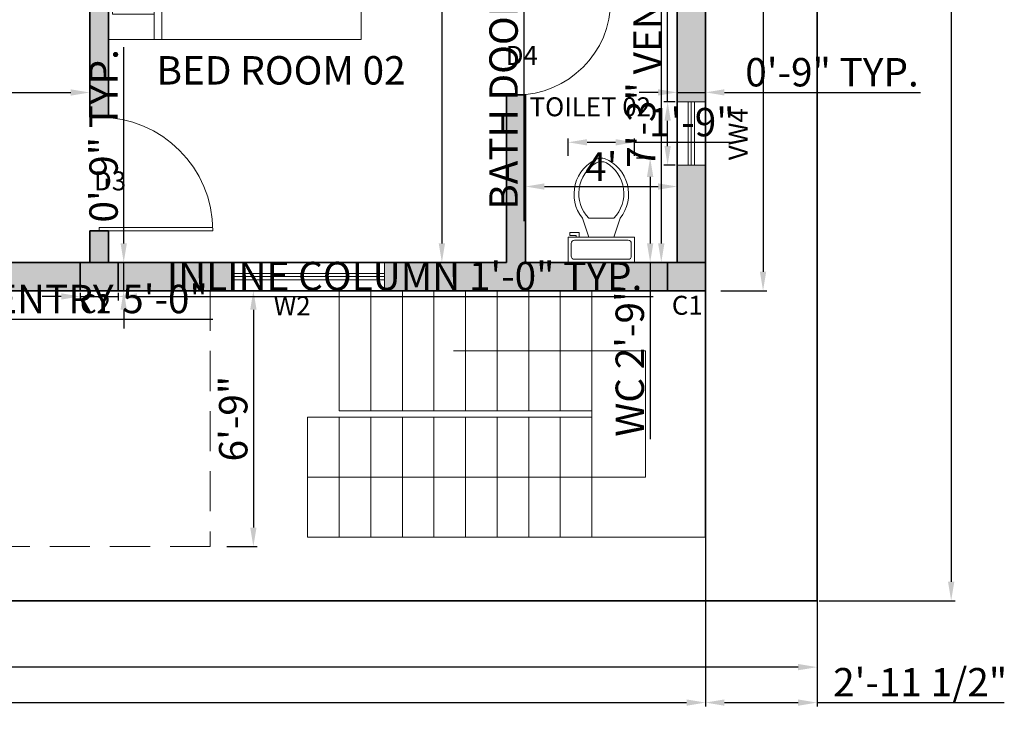
# Model space of a CAD drawing. Units: inches. Extents: x 4312 to 4955, y 6030 to 6717.
# Tile 2 of 5: x 4643 to 4955, y 6030 to 6255. Entities that reach past the tile are written whole.
import ezdxf

# ---------------------------------------------------------------- set-up
doc = ezdxf.new("R2010")
doc.units = ezdxf.units.IN
doc.linetypes.add('DASHED', pattern=[19.05, 12.7, -6.35])
for name, color, linetype, lineweight in [('A-AREA-IDEN', 7, 'Continuous', 20), ('A-FLOR-FIXT', 9, 'Continuous', 18), ('A-FLOR-OVHD', 6, 'DASHED', 13), ('A-WALL', 7, 'Continuous', 35), ('C-PROP', 7, 'Continuous', 35), ('Dimensions', 112, 'Continuous', 13), ('Doors', 10, 'Continuous', 18), ('Furniture', 30, 'Continuous', 18), ('stair case', 130, 'Continuous', 18), ('Text', 30, 'Continuous', 18), ('Windows', 160, 'Continuous', 18)]:
    doc.layers.add(name, color=color, linetype=linetype, lineweight=lineweight)
doc.layers.add('A-WALL-PATT', color=251, linetype='Continuous', lineweight=13, true_color=0x636466)
doc.layers.add('Column', color=52, linetype='Continuous', lineweight=35, true_color=0xc8c92d)
doc.styles.get("Standard").update_dxf_attribs({"font": 'arial.ttf'})
doc.dimstyles.new('ISO-25', dxfattribs={"dimtxt": 9, "dimasz": 6, "dimexe": 1.25, "dimexo": 0.625, "dimtad": 1, "dimdec": 1, "dimlunit": 3, "dimtxsty": 'Standard', "dimcen": 2.5, "dimadec": 0, "dimazin": 0, "dimtfac": 1, "dimtdec": 1, "dimtmove": 0, "dimatfit": 3, "dimfxl": 1, "dimarcsym": 0})

# ---------------------------------------------------------------- blocks, each defined once
blk = doc.blocks.new('D2')
at = {"layer": 'Doors'}
for p, q in [((4718.9, 6093.56), (4754.9, 6093.56)), ((4718.9, 6092.56), (4718.9, 6093.56)), ((4718.9, 6092.56), (4754.9, 6092.56))]:
    blk.add_line(p, q, dxfattribs=at)
blk.add_arc((4718.9, 6092.56), 36, 0, 90, dxfattribs=at)
blk = doc.blocks.new('D3')
at = {"layer": 'Doors'}
for p, q in [((5099.4, 6188.56), (5129.4, 6188.56)), ((5099.4, 6187.72), (5099.4, 6188.56)), ((5099.4, 6187.72), (5129.4, 6187.72))]:
    blk.add_line(p, q, dxfattribs=at)
blk.add_arc((5099.4, 6187.72), 30, 0, 90, dxfattribs=at)
blk = doc.blocks.new('*D17')
at = {"layer": 'Defpoints', "color": 0, "transparency": 16777216}
for p in [(4846.78, 6264.72), (4846.03, 6177.72), (4846.78, 6177.72)]:
    blk.add_point(p, dxfattribs=at)
at = {"layer": 'Dimensions', "color": 0, "lineweight": -2, "transparency": 16777216}
for p, q in [((4846.16, 6264.72), (4844.78, 6264.72)), ((4846.03, 6258.72), (4846.03, 6183.72)), ((4846.16, 6177.72), (4844.78, 6177.72))]:
    blk.add_line(p, q, dxfattribs=at)
at = {"layer": 'Dimensions', "color": 0, "transparency": 16777216}
for points in [[(4845.03, 6258.72), (4847.03, 6258.72), (4846.03, 6264.72)], [(4845.03, 6183.72), (4847.03, 6183.72), (4846.03, 6177.72)]]:
    blk.add_solid(points, dxfattribs=at)
at = {"layer": 'Dimensions', "color": 0, "transparency": 16777216, "insert": (4840.81, 6221.22), "char_height": 9, "attachment_point": 5, "rotation": 90}
blk.add_mtext('7\'-3"', dxfattribs=at)
blk = doc.blocks.new('*D18')
at = {"layer": 'Defpoints', "color": 0, "transparency": 16777216}
for p in [(4803.05, 6207.81), (4851.05, 6207.81), (4851.05, 6201.73)]:
    blk.add_point(p, dxfattribs=at)
at = {"layer": 'Dimensions', "color": 0, "lineweight": -2, "transparency": 16777216}
for p, q in [((4803.05, 6207.19), (4803.05, 6200.48)), ((4851.05, 6207.19), (4851.05, 6200.48)), ((4809.05, 6201.73), (4845.05, 6201.73))]:
    blk.add_line(p, q, dxfattribs=at)
at = {"layer": 'Dimensions', "color": 0, "transparency": 16777216}
for points in [[(4809.05, 6202.73), (4809.05, 6200.73), (4803.05, 6201.73)], [(4845.05, 6202.73), (4845.05, 6200.73), (4851.05, 6201.73)]]:
    blk.add_solid(points, dxfattribs=at)
at = {"layer": 'Dimensions', "color": 0, "transparency": 16777216, "insert": (4827.05, 6206.86), "char_height": 9, "attachment_point": 5}
blk.add_mtext("4'", dxfattribs=at)
blk = doc.blocks.new('*D19')
at = {"layer": 'Defpoints', "color": 0, "transparency": 16777216}
for p in [(4774.62, 6357.72), (4774.62, 6177.72), (4776.57, 6177.72)]:
    blk.add_point(p, dxfattribs=at)
at = {"layer": 'Dimensions', "color": 0, "lineweight": -2, "transparency": 16777216}
for p, q in [((4775.24, 6357.72), (4777.82, 6357.72)), ((4776.57, 6351.72), (4776.57, 6183.72)), ((4775.24, 6177.72), (4777.82, 6177.72))]:
    blk.add_line(p, q, dxfattribs=at)
at = {"layer": 'Dimensions', "color": 0, "transparency": 16777216}
for points in [[(4775.57, 6351.72), (4777.57, 6351.72), (4776.57, 6357.72)], [(4775.57, 6183.72), (4777.57, 6183.72), (4776.57, 6177.72)]]:
    blk.add_solid(points, dxfattribs=at)
at = {"layer": 'Dimensions', "color": 0, "transparency": 16777216, "insert": (4771.35, 6267.72), "char_height": 9, "attachment_point": 5, "rotation": 90}
blk.add_mtext("15'", dxfattribs=at)
blk = doc.blocks.new('*D21')
at = {"layer": 'Defpoints', "color": 0, "transparency": 16777216}
for p in [(4425.05, 6231.5), (4665.05, 6231.5), (4665.05, 6231.5)]:
    blk.add_point(p, dxfattribs=at)
at = {"layer": 'Dimensions', "color": 0, "lineweight": -2, "transparency": 16777216}
for p, q in [((4425.05, 6232.12), (4425.05, 6232.75)), ((4665.05, 6232.12), (4665.05, 6232.75)), ((4431.05, 6231.5), (4659.05, 6231.5))]:
    blk.add_line(p, q, dxfattribs=at)
at = {"layer": 'Dimensions', "color": 0, "transparency": 16777216}
for points in [[(4431.05, 6232.5), (4431.05, 6230.5), (4425.05, 6231.5)], [(4659.05, 6232.5), (4659.05, 6230.5), (4665.05, 6231.5)]]:
    blk.add_solid(points, dxfattribs=at)
at = {"layer": 'Dimensions', "color": 0, "transparency": 16777216, "insert": (4545.05, 6236.72), "char_height": 9, "attachment_point": 5}
blk.add_mtext("20'", dxfattribs=at)
blk = doc.blocks.new('*D25')
at = {"layer": 'Defpoints', "color": 0, "transparency": 16777216}
for p in [(4707.84, 6168.72), (4707.84, 6087.72), (4716.88, 6087.72)]:
    blk.add_point(p, dxfattribs=at)
at = {"layer": 'Dimensions', "color": 0, "lineweight": -2, "transparency": 16777216}
for p, q in [((4708.47, 6168.72), (4718.13, 6168.72)), ((4716.88, 6162.72), (4716.88, 6093.72)), ((4708.47, 6087.72), (4718.13, 6087.72))]:
    blk.add_line(p, q, dxfattribs=at)
at = {"layer": 'Dimensions', "color": 0, "transparency": 16777216}
for points in [[(4715.88, 6162.72), (4717.88, 6162.72), (4716.88, 6168.72)], [(4715.88, 6093.72), (4717.88, 6093.72), (4716.88, 6087.72)]]:
    blk.add_solid(points, dxfattribs=at)
at = {"layer": 'Dimensions', "color": 0, "transparency": 16777216, "insert": (4711.66, 6128.22), "char_height": 9, "attachment_point": 5, "rotation": 90}
blk.add_mtext('6\'-9"', dxfattribs=at)
blk = doc.blocks.new('Toilet - top')
for p, q in [((9.5, -6), (9.5, -2)), ((-10, -8.5), (-8, -8.5)), ((-10, -9.5), (-10, -8.5)), ((-8, -8.5), (-8, -8)), ((-7, -8), (-7, -9.5)), ((-4, -8), (-6, -14)), ((4, -8), (6, -14)), ((-7, -9.5), (-10, -9.5)), ((4, -14), (-4, -14))]:
    blk.add_line(p, q)
blk.add_lwpolyline([(10.5, -8), (10.5, 0), (-10.5, 0), (-10.5, -8)], close=True)
for points in [[(-9.5, -2), (-9.5, -6)], [(8.5, -1), (-8.5, -1)], [(-8.5, -7), (8.5, -7)]]:
    blk.add_lwpolyline(points)
for centre, radius, start, end in [((-8.62, -1.88), 0.884, 81.8699, 188.1301), ((8.62, -1.88), 0.884, 351.8699, 98.1301), ((-8.62, -6.12), 0.884, 171.8699, 278.1301), ((8.62, -6.12), 0.884, 261.8699, 8.1301), ((3.52, -21.58), 12.17, 141.4691, 247.9714), ((4.2, -21.82), 11.33, 136.3677, 238.9468), ((-3.52, -21.58), 12.17, 292.0284, 38.5307), ((-4.2, -21.82), 11.33, 301.053, 43.6321), ((0, -27.88), 4, 245.7318, 294.2682), ((0, -29), 4, 254.8605, 285.1395)]:
    blk.add_arc(centre, radius, start, end)
blk = doc.blocks.new('*D39')
at = {"layer": 'Defpoints', "color": 0, "transparency": 16777216}
for p in [(4857.98, 6552.72), (4864.3, 6168.72), (4878.26, 6168.72)]:
    blk.add_point(p, dxfattribs=at)
at = {"layer": 'Dimensions', "color": 0, "lineweight": -2, "transparency": 16777216}
for p, q in [((4858.6, 6552.72), (4879.51, 6552.72)), ((4878.26, 6546.72), (4878.26, 6174.72)), ((4864.93, 6168.72), (4879.51, 6168.72))]:
    blk.add_line(p, q, dxfattribs=at)
at = {"layer": 'Dimensions', "color": 0, "transparency": 16777216}
for points in [[(4877.26, 6546.72), (4879.26, 6546.72), (4878.26, 6552.72)], [(4877.26, 6174.72), (4879.26, 6174.72), (4878.26, 6168.72)]]:
    blk.add_solid(points, dxfattribs=at)
at = {"layer": 'Dimensions', "color": 0, "transparency": 16777216, "insert": (4873.03, 6360.72), "char_height": 9, "attachment_point": 5, "rotation": 90}
blk.add_mtext("32'", dxfattribs=at)
blk = doc.blocks.new('*D41')
at = {"layer": 'Defpoints', "color": 0, "transparency": 16777216}
for p in [(4895.36, 6639.55), (4895.36, 6070.55), (4937.83, 6070.55)]:
    blk.add_point(p, dxfattribs=at)
at = {"layer": 'Dimensions', "color": 0, "lineweight": -2, "transparency": 16777216}
for p, q in [((4895.99, 6639.55), (4939.08, 6639.55)), ((4937.83, 6633.55), (4937.83, 6076.55)), ((4895.99, 6070.55), (4939.08, 6070.55))]:
    blk.add_line(p, q, dxfattribs=at)
at = {"layer": 'Dimensions', "color": 0, "transparency": 16777216}
for points in [[(4936.83, 6633.55), (4938.83, 6633.55), (4937.83, 6639.55)], [(4936.83, 6076.55), (4938.83, 6076.55), (4937.83, 6070.55)]]:
    blk.add_solid(points, dxfattribs=at)
at = {"layer": 'Dimensions', "color": 0, "transparency": 16777216, "insert": (4931.11, 6355.05), "char_height": 12, "attachment_point": 5, "rotation": 90}
blk.add_mtext('47\'-5"', dxfattribs=at)
blk = doc.blocks.new('*D42')
at = {"layer": 'Defpoints', "color": 0, "transparency": 16777216}
for p in [(4355.36, 6070.55), (4895.36, 6070.55), (4355.36, 6049.53)]:
    blk.add_point(p, dxfattribs=at)
at = {"layer": 'Dimensions', "color": 0, "lineweight": -2, "transparency": 16777216}
for p, q in [((4355.36, 6069.92), (4355.36, 6048.28)), ((4895.36, 6069.92), (4895.36, 6048.28)), ((4889.36, 6049.53), (4361.36, 6049.53))]:
    blk.add_line(p, q, dxfattribs=at)
at = {"layer": 'Dimensions', "color": 0, "transparency": 16777216}
for points in [[(4361.36, 6050.53), (4361.36, 6048.53), (4355.36, 6049.53)], [(4889.36, 6050.53), (4889.36, 6048.53), (4895.36, 6049.53)]]:
    blk.add_solid(points, dxfattribs=at)
at = {"layer": 'Dimensions', "color": 0, "transparency": 16777216, "insert": (4625.36, 6056.26), "char_height": 12, "attachment_point": 5}
blk.add_mtext("45'", dxfattribs=at)
blk = doc.blocks.new('BED-QUEEN-PLAN')
for p, q in [((0, 0), (0, 80.00003)), ((7.99999, 78.80003), (28.79998, 78.80003)), ((7.99999, 65.60003), (7.99999, 78.80003)), ((28.79998, 78.80003), (28.79998, 65.60003)), ((31.19999, 78.80003), (51.99999, 78.80003)), ((31.19999, 65.60003), (31.19999, 78.80003)), ((51.99999, 78.80003), (51.99999, 63.60003)), ((59.99999, 80.00003), (59.99999, 0)), ((0, 65.60003), (44.8, 65.60003)), ((59.99999, 50.40003), (44.8, 65.60003)), ((44.8, 65.60003), (44.8, 50.40003)), ((44.8, 63.20003), (0, 63.20003)), ((51.99999, 63.60003), (46.79936, 63.60003)), ((44.8, 50.40003), (59.99999, 50.40003)), ((59.99999, 0), (0, 0))]:
    blk.add_line(p, q)
blk = doc.blocks.new('VENT-WINDOW-20')
for p, q in [((0, 20), (9, 20)), ((3.5, 20), (3.5, 0)), ((4.5, 20), (4.5, 0)), ((5.5, 20), (5.5, 0)), ((9, 0), (0, 0))]:
    blk.add_line(p, q)
blk = doc.blocks.new('COLUMN-12X9-INLINE')
h = blk.add_hatch(color=256)
h.dxf.hatch_style = 1
h.paths.add_polyline_path([(12, 0), (12, 9), (0, 9), (0, 0)])
for points in [[(0, 0), (0, 9)], [(12, 9), (12, 0)]]:
    blk.add_lwpolyline(points)
blk = doc.blocks.new('*D55')
at = {"layer": 'Defpoints', "color": 0, "transparency": 16777216}
for p in [(4662.02, 6168.72), (4674.02, 6168.72), (4674.02, 6166.92)]:
    blk.add_point(p, dxfattribs=at)
at = {"layer": 'Dimensions', "color": 0, "lineweight": -2, "transparency": 16777216}
for p, q in [((4656.02, 6166.92), (4650.02, 6166.92)), ((4662.02, 6168.1), (4662.02, 6165.67)), ((4662.02, 6166.92), (4674.02, 6166.92)), ((4674.02, 6168.1), (4674.02, 6165.67)), ((4680.02, 6166.92), (4843.47, 6166.92))]:
    blk.add_line(p, q, dxfattribs=at)
at = {"layer": 'Dimensions', "color": 0, "transparency": 16777216}
for points in [[(4656.02, 6167.92), (4656.02, 6165.92), (4662.02, 6166.92)], [(4680.02, 6167.92), (4680.02, 6165.92), (4674.02, 6166.92)]]:
    blk.add_solid(points, dxfattribs=at)
at = {"layer": 'Dimensions', "color": 0, "transparency": 16777216, "insert": (4764.74, 6172.21), "char_height": 9, "attachment_point": 5}
blk.add_mtext('INLINE COLUMN 1\'-0" TYP.', dxfattribs=at)
blk = doc.blocks.new('*D56')
at = {"layer": 'Defpoints', "color": 0, "transparency": 16777216}
for p in [(4674.02, 6177.72), (4675.82, 6177.72), (4674.02, 6168.72)]:
    blk.add_point(p, dxfattribs=at)
at = {"layer": 'Dimensions', "color": 0, "lineweight": -2, "transparency": 16777216}
for p, q in [((4675.82, 6183.72), (4675.82, 6245.83)), ((4674.64, 6177.72), (4677.07, 6177.72)), ((4675.82, 6168.72), (4675.82, 6177.72)), ((4674.64, 6168.72), (4677.07, 6168.72)), ((4675.82, 6162.72), (4675.82, 6156.72))]:
    blk.add_line(p, q, dxfattribs=at)
at = {"layer": 'Dimensions', "color": 0, "transparency": 16777216}
for points in [[(4674.82, 6183.72), (4676.82, 6183.72), (4675.82, 6177.72)], [(4674.82, 6162.72), (4676.82, 6162.72), (4675.82, 6168.72)]]:
    blk.add_solid(points, dxfattribs=at)
at = {"layer": 'Dimensions', "color": 0, "transparency": 16777216, "insert": (4670.6, 6217.78), "char_height": 9, "attachment_point": 5, "rotation": 90}
blk.add_mtext('0\'-9" TYP.', dxfattribs=at)
blk = doc.blocks.new('*D61')
at = {"layer": 'Defpoints', "color": 0, "transparency": 16777216}
for p in [(4807.05, 6360.72), (4802.55, 6330.72), (4807.05, 6330.72)]:
    blk.add_point(p, dxfattribs=at)
at = {"layer": 'Dimensions', "color": 0, "lineweight": -2, "transparency": 16777216}
for p, q in [((4806.42, 6360.72), (4801.3, 6360.72)), ((4802.55, 6354.72), (4802.55, 6336.72)), ((4806.42, 6330.72), (4801.3, 6330.72)), ((4802.55, 6330.72), (4802.55, 6190.78))]:
    blk.add_line(p, q, dxfattribs=at)
at = {"layer": 'Dimensions', "color": 0, "transparency": 16777216}
for points in [[(4801.55, 6354.72), (4803.55, 6354.72), (4802.55, 6360.72)], [(4801.55, 6336.72), (4803.55, 6336.72), (4802.55, 6330.72)]]:
    blk.add_solid(points, dxfattribs=at)
at = {"layer": 'Dimensions', "color": 0, "transparency": 16777216, "insert": (4797.27, 6257.75), "char_height": 9, "attachment_point": 5, "rotation": 90}
blk.add_mtext('BATH DOOR 2\'-6" TYP.', dxfattribs=at)
blk = doc.blocks.new('*D65')
at = {"layer": 'Defpoints', "color": 0, "transparency": 16777216}
for p in [(4848.05, 6228.54), (4851.05, 6228.54), (4851.05, 6208.54)]:
    blk.add_point(p, dxfattribs=at)
at = {"layer": 'Dimensions', "color": 0, "lineweight": -2, "transparency": 16777216}
for p, q in [((4848.05, 6228.54), (4848.05, 6328.15)), ((4850.42, 6228.54), (4846.8, 6228.54)), ((4848.05, 6214.54), (4848.05, 6222.54)), ((4850.42, 6208.54), (4846.8, 6208.54))]:
    blk.add_line(p, q, dxfattribs=at)
at = {"layer": 'Dimensions', "color": 0, "transparency": 16777216}
for points in [[(4847.05, 6222.54), (4849.05, 6222.54), (4848.05, 6228.54)], [(4847.05, 6214.54), (4849.05, 6214.54), (4848.05, 6208.54)]]:
    blk.add_solid(points, dxfattribs=at)
at = {"layer": 'Dimensions', "color": 0, "transparency": 16777216, "insert": (4842.83, 6281.35), "char_height": 9, "attachment_point": 5, "rotation": 90}
blk.add_mtext('VENT 1\'-8" TYP.', dxfattribs=at)
blk = doc.blocks.new('*D66')
at = {"layer": 'Defpoints', "color": 0, "transparency": 16777216}
for p in [(4860.05, 6231.54), (4851.05, 6228.54), (4860.05, 6228.54)]:
    blk.add_point(p, dxfattribs=at)
at = {"layer": 'Dimensions', "color": 0, "lineweight": -2, "transparency": 16777216}
for p, q in [((4851.05, 6229.17), (4851.05, 6232.79)), ((4860.05, 6229.17), (4860.05, 6232.79)), ((4845.05, 6231.54), (4839.05, 6231.54)), ((4851.05, 6231.54), (4860.05, 6231.54)), ((4866.05, 6231.54), (4928.16, 6231.54))]:
    blk.add_line(p, q, dxfattribs=at)
at = {"layer": 'Dimensions', "color": 0, "transparency": 16777216}
for points in [[(4845.05, 6232.54), (4845.05, 6230.54), (4851.05, 6231.54)], [(4866.05, 6232.54), (4866.05, 6230.54), (4860.05, 6231.54)]]:
    blk.add_solid(points, dxfattribs=at)
at = {"layer": 'Dimensions', "color": 0, "transparency": 16777216, "insert": (4900.1, 6236.76), "char_height": 9, "attachment_point": 5}
blk.add_mtext('0\'-9" TYP.', dxfattribs=at)
blk = doc.blocks.new('*D67')
at = {"layer": 'Defpoints', "color": 0, "transparency": 16777216}
for p in [(4567.22, 6168.72), (4627.22, 6168.72), (4627.22, 6159.72)]:
    blk.add_point(p, dxfattribs=at)
at = {"layer": 'Dimensions', "color": 0, "lineweight": -2, "transparency": 16777216}
for p, q in [((4567.22, 6168.1), (4567.22, 6158.47)), ((4627.22, 6168.1), (4627.22, 6158.47)), ((4573.22, 6159.72), (4621.22, 6159.72)), ((4627.22, 6159.72), (4704.03, 6159.72))]:
    blk.add_line(p, q, dxfattribs=at)
at = {"layer": 'Dimensions', "color": 0, "transparency": 16777216}
for points in [[(4573.22, 6160.72), (4573.22, 6158.72), (4567.22, 6159.72)], [(4621.22, 6160.72), (4621.22, 6158.72), (4627.22, 6159.72)]]:
    blk.add_solid(points, dxfattribs=at)
at = {"layer": 'Dimensions', "color": 0, "transparency": 16777216, "insert": (4668.63, 6164.94), "char_height": 9, "attachment_point": 5}
blk.add_mtext('ENTRY 5\'-0"', dxfattribs=at)
blk = doc.blocks.new('*D68')
at = {"layer": 'Defpoints', "color": 0, "transparency": 16777216}
for p in [(4627.22, 6202.22), (4636.22, 6202.22), (4627.22, 6168.72)]:
    blk.add_point(p, dxfattribs=at)
at = {"layer": 'Dimensions', "color": 0, "lineweight": -2, "transparency": 16777216}
for p, q in [((4636.22, 6202.22), (4636.22, 6254.52)), ((4627.85, 6202.22), (4637.47, 6202.22)), ((4636.22, 6174.72), (4636.22, 6196.22)), ((4627.85, 6168.72), (4637.47, 6168.72))]:
    blk.add_line(p, q, dxfattribs=at)
at = {"layer": 'Dimensions', "color": 0, "transparency": 16777216}
for points in [[(4635.22, 6196.22), (4637.22, 6196.22), (4636.22, 6202.22)], [(4635.22, 6174.72), (4637.22, 6174.72), (4636.22, 6168.72)]]:
    blk.add_solid(points, dxfattribs=at)
at = {"layer": 'Dimensions', "color": 0, "transparency": 16777216, "insert": (4630.94, 6231.37), "char_height": 9, "attachment_point": 5, "rotation": 90}
blk.add_mtext('2\'-9 1/2"', dxfattribs=at)
blk = doc.blocks.new('*D85')
at = {"layer": 'Defpoints', "color": 0, "transparency": 16777216}
for p in [(4837.55, 6210.77), (4837.55, 6177.72), (4842.51, 6177.72)]:
    blk.add_point(p, dxfattribs=at)
at = {"layer": 'Dimensions', "color": 0, "lineweight": -2, "transparency": 16777216}
for p, q in [((4838.17, 6210.77), (4843.76, 6210.77)), ((4842.51, 6204.77), (4842.51, 6183.72)), ((4838.17, 6177.72), (4843.76, 6177.72)), ((4842.51, 6177.72), (4842.51, 6121.74))]:
    blk.add_line(p, q, dxfattribs=at)
at = {"layer": 'Dimensions', "color": 0, "transparency": 16777216}
for points in [[(4841.51, 6204.77), (4843.51, 6204.77), (4842.51, 6210.77)], [(4841.51, 6183.72), (4843.51, 6183.72), (4842.51, 6177.72)]]:
    blk.add_solid(points, dxfattribs=at)
at = {"layer": 'Dimensions', "color": 0, "transparency": 16777216, "insert": (4837.23, 6146.73), "char_height": 9, "attachment_point": 5, "rotation": 90}
blk.add_mtext('WC 2\'-9"', dxfattribs=at)
blk = doc.blocks.new('*D86')
at = {"layer": 'Defpoints', "color": 0, "transparency": 16777216}
for p in [(4837.55, 6215.73), (4816.55, 6210.77), (4837.55, 6210.77)]:
    blk.add_point(p, dxfattribs=at)
at = {"layer": 'Dimensions', "color": 0, "lineweight": -2, "transparency": 16777216}
for p, q in [((4816.55, 6211.4), (4816.55, 6216.98)), ((4837.55, 6211.4), (4837.55, 6216.98)), ((4822.55, 6215.73), (4831.55, 6215.73)), ((4837.55, 6215.73), (4867.88, 6215.73))]:
    blk.add_line(p, q, dxfattribs=at)
at = {"layer": 'Dimensions', "color": 0, "transparency": 16777216}
for points in [[(4822.55, 6216.73), (4822.55, 6214.73), (4816.55, 6215.73)], [(4831.55, 6216.73), (4831.55, 6214.73), (4837.55, 6215.73)]]:
    blk.add_solid(points, dxfattribs=at)
at = {"layer": 'Dimensions', "color": 0, "transparency": 16777216, "insert": (4855.71, 6220.95), "char_height": 9, "attachment_point": 5}
blk.add_mtext('1\'-9"', dxfattribs=at)
blk = doc.blocks.new('*D88')
at = {"layer": 'Defpoints', "color": 0, "transparency": 16777216}
for p in [(4895.36, 6639.55), (4860.05, 6552.72), (4895.36, 6038.3)]:
    blk.add_point(p, dxfattribs=at)
at = {"layer": 'Dimensions', "color": 0, "lineweight": -2, "transparency": 16777216}
for p, q in [((4895.36, 6638.92), (4895.36, 6037.05)), ((4860.05, 6552.1), (4860.05, 6037.05)), ((4866.05, 6038.3), (4889.36, 6038.3)), ((4895.36, 6038.3), (4954.65, 6038.3))]:
    blk.add_line(p, q, dxfattribs=at)
at = {"layer": 'Dimensions', "color": 0, "transparency": 16777216}
for points in [[(4866.05, 6039.3), (4866.05, 6037.3), (4860.05, 6038.3)], [(4889.36, 6039.3), (4889.36, 6037.3), (4895.36, 6038.3)]]:
    blk.add_solid(points, dxfattribs=at)
at = {"layer": 'Dimensions', "color": 0, "transparency": 16777216, "insert": (4928.01, 6043.58), "char_height": 9, "attachment_point": 5}
blk.add_mtext('2\'-11 1/2"', dxfattribs=at)
blk = doc.blocks.new('*D89')
at = {"layer": 'Defpoints', "color": 0, "transparency": 16777216}
for p in [(4860.05, 6090.72), (4368.05, 6087.72), (4860.05, 6038.3)]:
    blk.add_point(p, dxfattribs=at)
at = {"layer": 'Dimensions', "color": 0, "lineweight": -2, "transparency": 16777216}
for p, q in [((4860.05, 6090.1), (4860.05, 6037.05)), ((4368.05, 6087.1), (4368.05, 6037.05)), ((4374.05, 6038.3), (4854.05, 6038.3))]:
    blk.add_line(p, q, dxfattribs=at)
at = {"layer": 'Dimensions', "color": 0, "transparency": 16777216}
for points in [[(4374.05, 6039.3), (4374.05, 6037.3), (4368.05, 6038.3)], [(4854.05, 6039.3), (4854.05, 6037.3), (4860.05, 6038.3)]]:
    blk.add_solid(points, dxfattribs=at)
at = {"layer": 'Dimensions', "color": 0, "transparency": 16777216, "insert": (4614.05, 6043.52), "char_height": 9, "attachment_point": 5}
blk.add_mtext('41\'-0"', dxfattribs=at)

msp = doc.modelspace()

# ---------------------------------------------------------------- hatches: boundary and pattern name
at = {"layer": 'A-WALL-PATT'}
h = msp.add_hatch(color=256, dxfattribs=at)
h.dxf.hatch_style = 1
h.paths.add_polyline_path([(4860.05, 6309.06), (4851.05, 6309.06), (4851.05, 6270.72), (4803.05, 6270.72), (4803.05, 6357.72), (4807.05, 6357.72), (4807.05, 6363.72), (4674.05, 6363.72), (4674.05, 6357.72), (4797.05, 6357.72), (4797.05, 6260.72), (4803.05, 6260.72), (4803.05, 6264.72), (4851.05, 6264.72), (4851.05, 6228.54), (4860.05, 6228.54)])
h = msp.add_hatch(color=256, dxfattribs=at)
h.dxf.hatch_style = 1
h.paths.add_polyline_path([(4671.05, 6351.72), (4665.05, 6351.72), (4665.05, 6223.72), (4671.05, 6223.72)])
h = msp.add_hatch(color=256, dxfattribs=at)
h.dxf.hatch_style = 1
h.paths.add_polyline_path([(4848.05, 6177.72), (4803.05, 6177.72), (4803.05, 6230.72), (4797.05, 6230.72), (4797.05, 6177.72), (4758.43, 6177.72), (4758.43, 6168.72), (4848.05, 6168.72)])
h = msp.add_hatch(color=256, dxfattribs=at)
h.dxf.hatch_style = 1
h.paths.add_polyline_path([(4860.05, 6208.54), (4851.05, 6208.54), (4851.05, 6177.72), (4860.05, 6177.72)])
h = msp.add_hatch(color=256, dxfattribs=at)
h.dxf.hatch_style = 1
h.paths.add_polyline_path([(4671.05, 6187.72), (4668.05, 6187.72), (4665.05, 6187.72), (4665.05, 6177.72), (4671.05, 6177.72)])
h = msp.add_hatch(color=256, dxfattribs=at)
h.dxf.hatch_style = 1
h.paths.add_polyline_path([(4662.02, 6177.72), (4627.22, 6177.72), (4627.22, 6168.72), (4662.02, 6168.72)])
h = msp.add_hatch(color=256, dxfattribs=at)
h.dxf.hatch_style = 1
h.paths.add_polyline_path([(4710.44, 6177.72), (4674.02, 6177.72), (4674.02, 6168.72), (4710.44, 6168.72)])
at = {"layer": 'Column'}
h = msp.add_hatch(color=256, dxfattribs=at)
h.dxf.hatch_style = 1
h.paths.add_polyline_path([(4860.05, 6168.72), (4860.05, 6177.72), (4848.05, 6177.72), (4848.05, 6168.72)])

# ---------------------------------------------------------------- linework, layer by layer
at = {"layer": 'A-FLOR-OVHD'}
for p, q in [((4703.23, 6168.72), (4703.23, 6087.72)), ((4703.23, 6087.72), (4368.05, 6087.72))]:
    msp.add_line(p, q, dxfattribs=at)
at = {"layer": 'A-WALL'}
for p, q in [((4860.05, 6552.72), (4860.05, 6090.72)), ((4665.05, 6367.72), (4665.05, 6223.72)), ((4671.05, 6357.72), (4671.05, 6223.72)), ((4851.05, 6264.72), (4851.05, 6177.72)), ((4797.05, 6230.72), (4803.05, 6230.72)), ((4797.05, 6230.72), (4797.05, 6177.72)), ((4803.05, 6230.72), (4803.05, 6177.72)), ((4671.05, 6223.72), (4665.05, 6223.72)), ((4671.05, 6187.72), (4665.05, 6187.72)), ((4665.05, 6187.72), (4665.05, 6177.72)), ((4671.05, 6187.72), (4671.05, 6177.72)), ((4797.05, 6177.72), (4627.22, 6177.72)), ((4797.05, 6177.72), (4671.05, 6177.72)), ((4851.05, 6177.72), (4803.05, 6177.72)), ((4860.05, 6168.72), (4416.05, 6168.72)), ((4860.05, 6168.72), (4627.22, 6168.72))]:
    msp.add_line(p, q, dxfattribs=at)
at = {"layer": 'C-PROP'}
msp.add_lwpolyline([(4895.36, 6639.55), (4895.36, 6070.55), (4355.36, 6070.55), (4379.36, 6639.55)], close=True, dxfattribs=at)
at = {"layer": 'Column'}
msp.add_lwpolyline([(4848.05, 6168.72), (4848.05, 6177.72), (4860.05, 6177.72)], dxfattribs=at)
at = {"layer": 'stair case'}
for p, q in [((4744.05, 6168.72), (4744.05, 6130.72)), ((4754.05, 6168.72), (4754.05, 6130.72)), ((4764.05, 6168.72), (4764.05, 6130.72)), ((4774.05, 6168.72), (4774.05, 6130.72)), ((4784.05, 6168.72), (4784.05, 6130.72)), ((4794.05, 6168.72), (4794.05, 6130.72)), ((4804.05, 6168.72), (4804.05, 6130.72)), ((4814.05, 6168.72), (4814.05, 6130.72)), ((4824.05, 6168.72), (4824.05, 6090.72)), ((4841.01, 6149.72), (4780.25, 6149.72)), ((4841.01, 6149.72), (4841.01, 6109.72)), ((4824.05, 6130.72), (4744.05, 6130.72)), ((4734.05, 6128.72), (4734.05, 6090.72)), ((4824.05, 6128.72), (4734.05, 6128.72)), ((4744.05, 6128.72), (4744.05, 6090.72)), ((4754.05, 6128.72), (4754.05, 6090.72)), ((4764.05, 6128.72), (4764.05, 6090.72)), ((4774.05, 6128.72), (4774.05, 6090.72)), ((4784.05, 6128.72), (4784.05, 6090.72)), ((4794.05, 6128.72), (4794.05, 6090.72)), ((4804.05, 6128.72), (4804.05, 6090.72)), ((4814.05, 6128.72), (4814.05, 6090.72)), ((4734.05, 6109.72), (4841.01, 6109.72)), ((4734.05, 6090.72), (4860.05, 6090.72))]:
    msp.add_line(p, q, dxfattribs=at)
at = {"layer": 'Windows'}
for p, q in [((4710.44, 6168.72), (4710.44, 6177.72)), ((4758.43, 6177.72), (4758.43, 6168.72)), ((4710.43, 6174.22), (4758.43, 6174.22)), ((4710.43, 6173.22), (4758.43, 6173.22)), ((4710.43, 6172.22), (4758.43, 6172.22))]:
    msp.add_line(p, q, dxfattribs=at)

# ---------------------------------------------------------------- block references
at = {"layer": 'A-FLOR-FIXT', "xscale": -1, "rotation": 180}
msp.add_blockref('Toilet - top', (4827.05, 6177.72), dxfattribs=at)
at = {"layer": 'Column'}
msp.add_blockref('COLUMN-12X9-INLINE', (4662.02, 6168.72), dxfattribs=at)
at = {"layer": 'Doors', "xscale": -1, "rotation": 180}
msp.add_blockref('D3', (-299.35, 12448.45), dxfattribs=at)
at = {"layer": 'Doors'}
msp.add_blockref('D2', (-50.85, 95.16), dxfattribs=at)
at = {"layer": 'Furniture', "rotation": 90.00000000000134}
msp.add_blockref('BED-QUEEN-PLAN', (4751.05, 6248.3), dxfattribs=at)
at = {"layer": 'Windows'}
msp.add_blockref('VENT-WINDOW-20', (4851.05, 6208.54), dxfattribs=at)

# ---------------------------------------------------------------- texts
at = {"layer": 'A-AREA-IDEN', "attachment_point": 1, "rotation": 0.0025}
for s, width, insert, char_height in [('BED ROOM 02', 89.0701, (4686.22, 6243.02), 9), ('TOILET 02', 65.4832, (4804.33, 6229.98), 6)]:
    msp.add_mtext_dynamic_manual_height_columns(s, width=width, gutter_width=12.5, heights=[0], dxfattribs=dict(at, insert=insert, char_height=char_height))
at = {"layer": 'Text', "char_height": 6, "attachment_point": 1}
for s, insert in [('D4', (4796.78, 6246.25)), ('D3', (4666.42, 6206.5)), ('C2', (4662.01, 6167.61)), ('W2', (4723.29, 6166.97)), ('C1', (4849.38, 6167.12))]:
    msp.add_mtext_dynamic_manual_height_columns(s, width=4.4911, gutter_width=12.5, heights=[0], dxfattribs=dict(at, insert=insert))
at = {"layer": 'Text', "insert": (4867.39, 6210.06), "char_height": 6, "attachment_point": 1, "rotation": 90}
msp.add_mtext_dynamic_manual_height_columns('VW4', width=19.9533, gutter_width=12.5, heights=[0], dxfattribs=at)

# ---------------------------------------------------------------- dimensions: what is measured, and where the dimension line sits
at = {"layer": 'Dimensions'}
for base, p1, p2, override, picture, middle in [((4895.36, 6038.3), (4860.05, 6552.72), (4895.36, 6639.55), {"dimdec": 1, "dimlfac": 1, "dimrnd": 0, "dimzin": 1, "dimdsep": 46, "dimlunit": 4, "dimfrac": 2}, '*D88', (4928.01, 6043.58)), ((4665.05, 6231.5), (4425.05, 6231.5), (4665.05, 6231.5), {"dimclrd": 0, "dimclre": 0, "dimclrt": 0}, '*D21', (4545.05, 6236.72)), ((4837.55, 6215.73), (4816.55, 6210.77), (4837.55, 6210.77), {"dimdec": 1, "dimlfac": 1, "dimrnd": 0, "dimzin": 1, "dimdsep": 46, "dimlunit": 4, "dimfrac": 2}, '*D86', (4855.71, 6220.95)), ((4851.05, 6201.73), (4803.05, 6207.81), (4851.05, 6207.81), {"dimclrd": 0, "dimclre": 0, "dimclrt": 0}, '*D18', (4827.05, 6206.86)), ((4860.05, 6038.3), (4368.05, 6087.72), (4860.05, 6090.72), {"dimdec": 1, "dimlfac": 1, "dimrnd": 0, "dimzin": 1, "dimdsep": 46, "dimlunit": 4, "dimfrac": 2}, '*D89', (4614.05, 6043.52)), ((4355.36, 6049.53), (4895.36, 6070.55), (4355.36, 6070.55), {"dimtxt": 12, "dimclrd": 0, "dimclre": 0, "dimclrt": 0}, '*D42', (4625.36, 6056.26))]:
    dim = msp.add_linear_dim(base=base, p1=p1, p2=p2, dimstyle='ISO-25', override=override, dxfattribs=at)
    dim.commit()
    dim.dimension.update_dxf_attribs({"geometry": picture, "text_midpoint": middle})
for base, p1, p2, override, picture, middle in [((4937.83, 6070.55), (4895.36, 6639.55), (4895.36, 6070.55), {"dimtxt": 12, "dimclrd": 0, "dimclre": 0, "dimclrt": 0}, '*D41', (4931.11, 6355.05)), ((4878.26, 6168.72), (4857.98, 6552.72), (4864.3, 6168.72), {"dimclrd": 0, "dimclre": 0, "dimclrt": 0}, '*D39', (4873.03, 6360.72)), ((4776.57, 6177.72), (4774.62, 6357.72), (4774.62, 6177.72), {"dimclrd": 0, "dimclre": 0, "dimclrt": 0}, '*D19', (4771.35, 6267.72)), ((4846.03, 6177.72), (4846.78, 6264.72), (4846.78, 6177.72), {"dimclrd": 0, "dimclre": 0, "dimclrt": 0}, '*D17', (4840.81, 6221.22)), ((4636.22, 6202.22), (4627.22, 6168.72), (4627.22, 6202.22), {"dimdec": 1, "dimlfac": 1, "dimrnd": 0, "dimzin": 1, "dimdsep": 46, "dimlunit": 4, "dimfrac": 2}, '*D68', (4630.94, 6231.37)), ((4716.88, 6087.72), (4707.84, 6168.72), (4707.84, 6087.72), {"dimclrd": 0, "dimclre": 0, "dimclrt": 0}, '*D25', (4711.66, 6128.22))]:
    dim = msp.add_linear_dim(base=base, p1=p1, p2=p2, angle=90, dimstyle='ISO-25', override=override, dxfattribs=at)
    dim.commit()
    dim.dimension.update_dxf_attribs({"geometry": picture, "text_midpoint": middle})
for base, p1, p2, angle, text, picture, middle in [((4802.55, 6330.72), (4807.05, 6360.72), (4807.05, 6330.72), 270, 'BATH DOOR <> TYP.', '*D61', (4797.27, 6257.75)), ((4848.05, 6228.54), (4851.05, 6208.54), (4851.05, 6228.54), 90, 'VENT <> TYP.', '*D65', (4842.83, 6281.35)), ((4675.82, 6177.72), (4674.02, 6168.72), (4674.02, 6177.72), 90, '<> TYP.', '*D56', (4670.6, 6217.78)), ((4842.5062, 6177.7244), (4837.5493, 6210.7707), (4837.5493, 6177.7244), 270, 'WC <>', '*D85', (4837.2277, 6146.7331))]:
    dim = msp.add_linear_dim(base=base, p1=p1, p2=p2, angle=angle, text=text, dimstyle='ISO-25', override={"dimdec": 1, "dimlfac": 1, "dimrnd": 0, "dimzin": 1, "dimdsep": 46, "dimlunit": 4, "dimfrac": 2}, dxfattribs=at)
    dim.commit()
    dim.dimension.update_dxf_attribs({"geometry": picture, "text_midpoint": middle})
for base, p1, p2, text, picture, middle in [((4860.05, 6231.54), (4851.05, 6228.54), (4860.05, 6228.54), '<> TYP.', '*D66', (4900.1, 6236.76)), ((4674.02, 6166.92), (4662.02, 6168.72), (4674.02, 6168.72), 'INLINE COLUMN <> TYP.', '*D55', (4764.74, 6172.21)), ((4627.22, 6159.72), (4567.22, 6168.72), (4627.22, 6168.72), 'ENTRY <>', '*D67', (4668.63, 6164.94))]:
    dim = msp.add_linear_dim(base=base, p1=p1, p2=p2, text=text, dimstyle='ISO-25', override={"dimdec": 1, "dimlfac": 1, "dimrnd": 0, "dimzin": 1, "dimdsep": 46, "dimlunit": 4, "dimfrac": 2}, dxfattribs=at)
    dim.commit()
    dim.dimension.update_dxf_attribs({"geometry": picture, "text_midpoint": middle})

doc.saveas('drawing.dxf')
